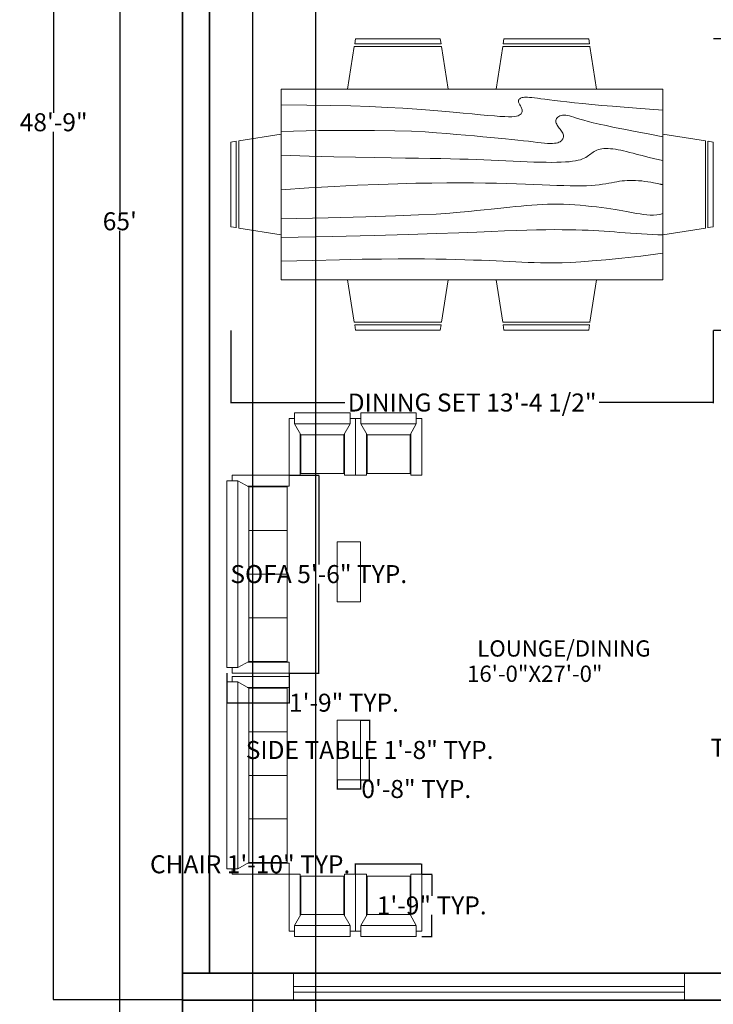
# Model space of a CAD drawing. Units: inches. Extents: x 79 to 8696167, y -3690578 to 147.
# Tile 2 of 10: x 79 to 310, y -551 to -223. Entities that reach past the tile are written whole.
import ezdxf

# ---------------------------------------------------------------- set-up
doc = ezdxf.new("R2010")
doc.units = ezdxf.units.IN
doc.header["$MEASUREMENT"] = 0
doc.layers.get('0').update_dxf_attribs({"color": 253})
for name, color, linetype, lineweight in [('A-ANNO-DIMS', 2, 'Continuous', 18), ('A-AREA-IDEN', 7, 'Continuous', 18), ('C-PROP', 7, 'Continuous', 35), ('furniture', 30, 'Continuous', 18), ('walls', 8, 'Continuous', 35), ('windows', 171, 'Continuous', 18)]:
    doc.layers.add(name, color=color, linetype=linetype, lineweight=lineweight)
doc.styles.get("Standard").update_dxf_attribs({"font": 'arial.ttf'})
doc.dimstyles.get("Standard").update_dxf_attribs({"dimtxt": 6, "dimasz": 0.18, "dimexe": 0.18, "dimexo": 0.0625, "dimgap": 0.09, "dimtad": 0, "dimtih": 1, "dimtoh": 1, "dimzin": 0, "dimdsep": 46, "dimlunit": 3, "dimtxsty": 'Standard', "dimcen": 0.09, "dimadec": 0, "dimazin": 0, "dimtfac": 1, "dimtofl": 0, "dimtmove": 0, "dimatfit": 3, "dimfxl": 1, "dimtolj": 1, "dimtzin": 0, "dimarcsym": 0})

# ---------------------------------------------------------------- blocks, each defined once
blk = doc.blocks.new('Dining Set - 36 x 72 in.')
for p, q in [((-22, 27.5), (-22.1562, 26.50042)), ((-5.8416, 26.5), (-22.1534, 26.5)), ((-22, 27.5), (-6, 27.5)), ((-5.8437, 26.49966), (-6, 27.5)), ((6, 27.5), (5.8438, 26.50042)), ((22.1584, 26.5), (5.8466, 26.5)), ((6, 27.5), (22, 27.5)), ((22.1563, 26.49966), (22, 27.5)), ((-22.2343, 26.00059), (-23.4847, 17.99762)), ((-22.2304, 26), (-5.7608, 26)), ((-4.5152, 17.99762), (-5.7655, 25.99926)), ((5.7657, 26.00059), (4.5153, 17.99762)), ((5.7696, 26), (22.2392, 26)), ((23.4848, 17.99762), (22.2345, 25.99926)), ((36, 18), (-36, 18)), ((-36, 18), (-36, -18)), ((36, -18), (36, 18)), ((-44.0006, 8.23428), (-35.9976, 9.48474)), ((44.0006, 8.23428), (35.9976, 9.48474)), ((-45.5, 8), (-44.5004, 8.15617)), ((-45.5, 8), (-45.5, -8)), ((-44.5, -8.15843), (-44.5, 8.15338)), ((-44, 8.23041), (-44, -8.23915)), ((44, 8.23041), (44, -8.23915)), ((44.5, -8.15843), (44.5, 8.15338)), ((45.5, 8), (44.5005, 8.15617)), ((45.5, 8), (45.5, -8)), ((-44.4997, -8.15631), (-45.5, -8)), ((-35.9976, -9.48476), (-43.9993, -8.2345)), ((35.9976, -9.48476), (43.9993, -8.2345)), ((44.4997, -8.15631), (45.5, -8)), ((-36, -18), (36, -18)), ((-22.2343, -26.0006), (-23.4847, -17.99762)), ((-4.5152, -17.99762), (-5.7655, -25.99928)), ((5.7657, -26.0006), (4.5153, -17.99762)), ((23.4848, -17.99762), (22.2345, -25.99928)), ((-22.2304, -26), (-5.7608, -26)), ((5.7696, -26), (22.2392, -26)), ((-22, -27.5), (-22.1562, -26.50044)), ((-5.8416, -26.5), (-22.1534, -26.5)), ((-22, -27.5), (-6, -27.5)), ((-5.8437, -26.49967), (-6, -27.5)), ((6, -27.5), (5.8438, -26.50044)), ((22.1584, -26.5), (5.8466, -26.5)), ((6, -27.5), (22, -27.5)), ((22.1563, -26.49967), (22, -27.5))]:
    blk.add_line(p, q)
for points in [[(-36, 15), (-31.1772, 14.97754), (-26.8079, 14.91406), (-22.8538, 14.81543), (-19.276, 14.6875), (-16.0362, 14.53613), (-13.0957, 14.36718), (-10.4159, 14.18652), (-7.9583, 14), (-5.6904, 13.81315), (-3.6035, 13.63021), (-1.6954, 13.45508), (0.0365, 13.29166), (1.5945, 13.14388), (2.9811, 13.01562), (4.1988, 12.9108), (5.25, 12.83333), (6.1393, 12.78613), (6.8802, 12.76823), (7.4883, 12.77767), (7.9792, 12.8125), (8.3685, 12.87077), (8.6719, 12.95052), (8.9049, 13.0498), (9.0833, 13.16666), (9.2205, 13.29899), (9.3216, 13.44401), (9.3895, 13.59879), (9.4271, 13.76041), (9.4373, 13.92594), (9.4232, 14.09245), (9.3875, 14.257), (9.3333, 14.41666), (9.2638, 14.56917), (9.1836, 14.71484), (9.0975, 14.85465), (9.0104, 14.98958), (8.9272, 15.1206), (8.8529, 15.2487), (8.7922, 15.37483), (8.75, 15.5), (8.7305, 15.62467), (8.7344, 15.74739), (8.7617, 15.86621), (8.8125, 15.97916), (8.8867, 16.08431), (8.9844, 16.17968), (9.1055, 16.26334), (9.25, 16.33333), (9.4189, 16.38802), (9.6172, 16.42708), (9.8506, 16.45052), (10.125, 16.45833), (10.4463, 16.45052), (10.8203, 16.42708), (11.2529, 16.38802), (11.75, 16.33333), (12.3184, 16.26318), (12.9694, 16.17838), (13.7151, 16.07991), (14.5677, 15.96875), (15.5395, 15.84586), (16.6426, 15.71224), (17.8893, 15.56884), (19.2917, 15.41666), (20.859, 15.25667), (22.5879, 15.08984), (24.4721, 14.91715), (26.5052, 14.73958), (28.6809, 14.5581), (30.9929, 14.3737), (33.4347, 14.18733), (36, 14)], [(-36, 10), (-28.9766, 10.14274), (-23.1725, 10.20442), (-18.4241, 10.19775), (-14.5677, 10.13541), (-11.4399, 10.03011), (-8.877, 9.89453), (-6.7154, 9.74137), (-4.7917, 9.58333), (-2.9698, 9.43082), (-1.2246, 9.28515), (0.4415, 9.14534), (2.026, 9.01041), (3.5266, 8.87939), (4.9408, 8.7513), (6.266, 8.62516), (7.5, 8.5), (8.6411, 8.37549), (9.6914, 8.2539), (10.6538, 8.13818), (11.5312, 8.03125), (12.3267, 7.93603), (13.043, 7.85547), (13.6831, 7.79248), (14.25, 7.75), (14.7471, 7.7303), (15.1797, 7.73307), (15.5537, 7.75732), (15.875, 7.80208), (16.1494, 7.86637), (16.3828, 7.94922), (16.5811, 8.04964), (16.75, 8.16666), (16.8944, 8.29915), (17.0143, 8.44531), (17.1089, 8.60319), (17.1771, 8.77083), (17.218, 8.94629), (17.2305, 9.1276), (17.2137, 9.31282), (17.1667, 9.5), (17.0895, 9.6875), (16.987, 9.875), (16.8649, 10.0625), (16.7292, 10.25), (16.5856, 10.4375), (16.4401, 10.625), (16.2985, 10.8125), (16.1667, 11), (16.05, 11.18733), (15.9518, 11.3737), (15.8752, 11.5581), (15.8229, 11.73958), (15.798, 11.91715), (15.8034, 12.08984), (15.842, 12.25667), (15.9167, 12.41666), (16.0295, 12.56836), (16.1784, 12.70833), (16.3605, 12.83268), (16.5729, 12.9375), (16.8127, 13.01888), (17.0768, 13.07291), (17.3625, 13.0957), (17.6667, 13.08333), (17.9894, 13.03312), (18.3418, 12.94726), (18.7382, 12.82918), (19.1927, 12.68229), (19.7195, 12.51001), (20.3327, 12.31575), (21.0465, 12.10294), (21.875, 11.875), (22.8357, 11.63354), (23.959, 11.37304), (25.2786, 11.08618), (26.8282, 10.76562), (28.6414, 10.40405), (30.752, 9.99414), (33.1936, 9.52856), (36, 9)], [(-36, 5.5), (-30.7157, 5.3348), (-26.069, 5.20963), (-21.9946, 5.11767), (-18.4271, 5.05208), (-15.3009, 5.00602), (-12.5508, 4.97265), (-10.1112, 4.94515), (-7.9167, 4.91666), (-5.909, 4.88167), (-4.0586, 4.83984), (-2.3429, 4.79215), (-0.7396, 4.73958), (0.7739, 4.6831), (2.22, 4.6237), (3.6213, 4.56233), (5, 4.5), (6.373, 4.43782), (7.7344, 4.3776), (9.0723, 4.32129), (10.375, 4.27083), (11.6309, 4.22819), (12.8281, 4.19531), (13.9551, 4.17415), (15, 4.16666), (15.954, 4.17448), (16.819, 4.19791), (17.6001, 4.23698), (18.3021, 4.29166), (18.9299, 4.36198), (19.4883, 4.44791), (19.9823, 4.54948), (20.4167, 4.66666), (20.7969, 4.79899), (21.1302, 4.94401), (21.4245, 5.09879), (21.6875, 5.26041), (21.9271, 5.42594), (22.1511, 5.59245), (22.3672, 5.757), (22.5834, 5.91666), (22.8065, 6.06868), (23.0404, 6.21093), (23.2879, 6.34147), (23.5521, 6.45833), (23.8358, 6.55957), (24.142, 6.64323), (24.4735, 6.70735), (24.8334, 6.75), (25.2235, 6.76969), (25.642, 6.76692), (26.0858, 6.74267), (26.5521, 6.69791), (27.0379, 6.63362), (27.5404, 6.55078), (28.0565, 6.45036), (28.5834, 6.33333), (29.1242, 6.19987), (29.7071, 6.04687), (30.3661, 5.87044), (31.1354, 5.66666), (32.0493, 5.43164), (33.142, 5.16146), (34.4475, 4.85221), (36, 4.5)], [(-36, -1), (-30.7915, -0.6591), (-26.0195, -0.38216), (-21.6519, -0.16284), (-17.6563, 0.00521), (-14.0005, 0.12833), (-10.6523, 0.21289), (-7.5796, 0.26522), (-4.75, 0.29166), (-2.134, 0.29793), (0.2878, 0.28711), (2.5317, 0.26163), (4.6146, 0.22396), (6.5529, 0.17651), (8.3633, 0.12174), (10.0623, 0.06209), (11.6667, 0), (13.1899, -0.06201), (14.6341, -0.1211), (15.9982, -0.17432), (17.2813, -0.21875), (18.4823, -0.25147), (19.6003, -0.26953), (20.6343, -0.27002), (21.5834, -0.25), (22.4481, -0.20768), (23.2357, -0.14584), (23.9549, -0.06836), (24.6146, 0.02083), (25.2235, 0.11784), (25.7904, 0.21875), (26.3241, 0.31966), (26.8334, 0.41666), (27.3265, 0.50618), (27.8099, 0.58593), (28.2894, 0.65397), (28.7709, 0.70833), (29.2601, 0.74707), (29.763, 0.76823), (30.2855, 0.76985), (30.8334, 0.75), (31.4088, 0.70784), (31.9994, 0.64713), (32.589, 0.57275), (33.1615, 0.48958), (33.7008, 0.4025), (34.1908, 0.3164), (34.6153, 0.23616), (34.9584, 0.16666), (35.2099, 0.11165), (35.3848, 0.07031), (35.504, 0.04069), (35.5886, 0.02083), (35.6594, 0.00879), (35.7377, 0.0026), (35.8442, 0.00032), (36, 0)], [(-36, -6.5), (-27.1843, -6.31267), (-20.084, -6.1263), (-14.469, -5.9419), (-10.1094, -5.76042), (-6.7752, -5.58285), (-4.2363, -5.41016), (-2.2629, -5.24333), (-0.625, -5.08334), (0.8708, -4.93099), (2.2715, -4.78646), (3.5872, -4.64974), (4.8281, -4.52084), (6.0046, -4.39974), (7.127, -4.28646), (8.2053, -4.18099), (9.25, -4.08334), (10.2705, -3.99382), (11.2734, -3.91407), (12.2647, -3.84603), (13.25, -3.79167), (14.2354, -3.75293), (15.2266, -3.73177), (16.2295, -3.73015), (17.25, -3.75), (18.2912, -3.79248), (19.3451, -3.85547), (20.4009, -3.93604), (21.4479, -4.03125), (22.4754, -4.13819), (23.4727, -4.25391), (24.4289, -4.37549), (25.3334, -4.5), (26.1785, -4.62492), (26.9694, -4.74935), (27.7145, -4.87281), (28.4219, -4.99479), (29.1, -5.11483), (29.7572, -5.23242), (30.4016, -5.34709), (31.0417, -5.45834), (31.6837, -5.56437), (32.3262, -5.65821), (32.9658, -5.73153), (33.599, -5.77604), (34.2224, -5.78345), (34.8327, -5.74545), (35.4264, -5.65373), (36, -5.5)], [(-36, -10), (-26.4022, -9.81299), (-18.4675, -9.62891), (-11.9839, -9.45069), (-6.7396, -9.28125), (-2.5226, -9.12354), (0.8789, -8.98047), (3.6769, -8.85498), (6.0833, -8.75), (8.2767, -8.66765), (10.3021, -8.60677), (12.1712, -8.56543), (13.8958, -8.54167), (15.4876, -8.53353), (16.9583, -8.53907), (18.3197, -8.55632), (19.5834, -8.58334), (20.7616, -8.61841), (21.8685, -8.66081), (22.9188, -8.71004), (23.9271, -8.76563), (24.9081, -8.82707), (25.8763, -8.89388), (26.8465, -8.96558), (27.8334, -9.04167), (28.8474, -9.12118), (29.8828, -9.20117), (30.93, -9.27824), (31.9792, -9.34896), (33.0205, -9.40991), (34.0443, -9.45768), (35.0407, -9.48885), (36, -9.5)], [(-36, -14.5), (-30.0881, -14.33513), (-25.0332, -14.21224), (-20.7312, -14.12647), (-17.0781, -14.07292), (-13.97, -14.04671), (-11.3027, -14.04297), (-8.9724, -14.05681), (-6.875, -14.08334), (-4.9224, -14.11833), (-3.0905, -14.16016), (-1.3709, -14.20785), (0.2448, -14.26042), (1.7647, -14.3169), (3.1973, -14.3763), (4.5507, -14.43767), (5.8333, -14.5), (7.0554, -14.5621), (8.235, -14.62175), (9.3922, -14.67652), (10.5469, -14.72396), (11.7192, -14.76164), (12.929, -14.78711), (14.1965, -14.79794), (15.5417, -14.79167), (16.9933, -14.76424), (18.6152, -14.70508), (20.4804, -14.60197), (22.6615, -14.44271), (25.2312, -14.21509), (28.2624, -13.9069), (31.8277, -13.50594), (36, -13)]]:
    blk.add_lwpolyline(points)
blk = doc.blocks.new('FABRIC SOFA 4S')
at = {"layer": 'furniture'}
for p, q in [((3, 54), (34, 54)), ((3, 51), (3, 54)), ((34, 48), (34, 54)), ((0, -51), (0, 51)), ((6, 51), (0, 51)), ((6, -51), (6, 51)), ((12, 47.63), (6, 51)), ((11.14, 48), (34, 48)), ((33, 23.81), (12, 23.81)), ((33, 0), (12, 0)), ((33, -23.81), (12, -23.81)), ((6, -51), (12, -47.63)), ((11.54, -48), (34, -48)), ((34, -48), (34, -54)), ((6, -51), (0, -51)), ((3, -54), (3, -51)), ((3, -54), (34, -54))]:
    blk.add_line(p, q, dxfattribs=at)
blk.add_lwpolyline([(12, -47.63), (12, 47.63), (33, 47.63), (33, -47.63)], close=True, dxfattribs=at)
blk = doc.blocks.new('FABRIC SOFA 1S')
at = {"layer": 'furniture'}
for p, q in [((3, 18.12), (34, 18.12)), ((3, 15.12), (3, 18.12)), ((34, 12.12), (34, 18.12)), ((0, -15.12), (0, 15.12)), ((6, 15.12), (0, 15.12)), ((6, -15.12), (6, 15.12)), ((12, 11.75), (6, 15.12)), ((11.33, 12.12), (34, 12.12)), ((6, -15.12), (0, -15.12)), ((3, -18.12), (3, -15.12)), ((6, -15.12), (12, -11.75)), ((11.33, -12.12), (34, -12.12)), ((34, -12.12), (34, -18.12)), ((3, -18.12), (34, -18.12))]:
    blk.add_line(p, q, dxfattribs=at)
blk.add_lwpolyline([(12, -11.75), (12, 11.75), (33, 11.75), (33, -11.75)], close=True, dxfattribs=at)
blk = doc.blocks.new('*D23')
at = {"layer": 'A-ANNO-DIMS', "color": 0, "lineweight": -2, "transparency": 16777216}
for p, q in [((133.38, 99.88), (112.4, 99.88)), ((112.58, 99.7), (112.58, -286.97)), ((112.58, -679.94), (112.58, -293.28)), ((133.38, -680.12), (112.4, -680.12))]:
    blk.add_line(p, q, dxfattribs=at)
at = {"layer": 'A-ANNO-DIMS', "color": 0, "lineweight": 100, "transparency": 16777216}
for points in [[(112.55, 99.7), (112.61, 99.7), (112.58, 99.88)], [(112.55, -679.94), (112.61, -679.94), (112.58, -680.12)]]:
    blk.add_solid(points, dxfattribs=at)
at = {"layer": 'Defpoints', "color": 0, "lineweight": 100, "transparency": 16777216}
for p in [(112.58, 99.88), (133.44, 99.88), (133.44, -680.12)]:
    blk.add_point(p, dxfattribs=at)
at = {"layer": 'A-ANNO-DIMS', "color": 0, "transparency": 16777216, "insert": (112.58, -290.12), "char_height": 6, "attachment_point": 5}
blk.add_mtext("\\A1;65'", dxfattribs=at)
blk = doc.blocks.new('TABLE-LOUNGE-NARROW')
for p, q in [((0, 19.98), (7.85, 19.98)), ((0, 0), (0, 19.98)), ((7.85, 19.98), (7.85, 0)), ((7.85, 0), (0, 0))]:
    blk.add_line(p, q)
blk = doc.blocks.new('*D33')
at = {"layer": 'A-ANNO-DIMS', "color": 0, "lineweight": -2, "transparency": 16777216}
for p, q in [((191.08, -504.4), (190.9, -504.4)), ((191.08, -507.66), (191.08, -504.22)), ((213.03, -504.4), (191.26, -504.4)), ((213.21, -507.66), (213.21, -504.22))]:
    blk.add_line(p, q, dxfattribs=at)
at = {"layer": 'A-ANNO-DIMS', "color": 0, "lineweight": 100, "transparency": 16777216}
for points in [[(191.26, -504.37), (191.26, -504.43), (191.08, -504.4)], [(213.03, -504.37), (213.03, -504.43), (213.21, -504.4)]]:
    blk.add_solid(points, dxfattribs=at)
at = {"layer": 'Defpoints', "color": 0, "lineweight": 100, "transparency": 16777216}
for p in [(191.08, -504.4), (191.08, -507.72), (213.21, -507.72)]:
    blk.add_point(p, dxfattribs=at)
at = {"layer": 'A-ANNO-DIMS', "color": 0, "transparency": 16777216, "insert": (156.02, -504.4), "char_height": 6, "attachment_point": 5}
blk.add_mtext('\\A1;CHAIR 1\'-10" TYP.', dxfattribs=at)
blk = doc.blocks.new('*D34')
at = {"layer": 'A-ANNO-DIMS', "color": 0, "lineweight": -2, "transparency": 16777216}
for p, q in [((213.27, -507.72), (216.71, -507.72)), ((216.53, -507.9), (216.53, -514.95)), ((216.53, -528.3), (216.53, -521.25)), ((213.27, -528.48), (216.71, -528.48))]:
    blk.add_line(p, q, dxfattribs=at)
at = {"layer": 'A-ANNO-DIMS', "color": 0, "lineweight": 100, "transparency": 16777216}
for points in [[(216.5, -507.9), (216.56, -507.9), (216.53, -507.72)], [(216.5, -528.3), (216.56, -528.3), (216.53, -528.48)]]:
    blk.add_solid(points, dxfattribs=at)
at = {"layer": 'Defpoints', "color": 0, "lineweight": 100, "transparency": 16777216}
for p in [(213.21, -507.72), (216.53, -507.72), (213.21, -528.48)]:
    blk.add_point(p, dxfattribs=at)
at = {"layer": 'A-ANNO-DIMS', "color": 0, "transparency": 16777216, "insert": (216.53, -518.1), "char_height": 6, "attachment_point": 5}
blk.add_mtext('\\A1;1\'-9" TYP.', dxfattribs=at)
blk = doc.blocks.new('*D35')
at = {"layer": 'A-ANNO-DIMS', "color": 0, "lineweight": -2, "transparency": 16777216}
for p, q in [((169.07, -374.73), (179.07, -374.73)), ((178.89, -374.91), (178.89, -404.5)), ((178.89, -440.48), (178.89, -410.89)), ((169.07, -440.66), (179.07, -440.66))]:
    blk.add_line(p, q, dxfattribs=at)
at = {"layer": 'A-ANNO-DIMS', "color": 0, "lineweight": 100, "transparency": 16777216}
for points in [[(178.86, -374.91), (178.92, -374.91), (178.89, -374.73)], [(178.86, -440.48), (178.92, -440.48), (178.89, -440.66)]]:
    blk.add_solid(points, dxfattribs=at)
at = {"layer": 'Defpoints', "color": 0, "lineweight": 100, "transparency": 16777216}
for p in [(169, -374.73), (178.89, -374.73), (169, -440.66)]:
    blk.add_point(p, dxfattribs=at)
at = {"layer": 'A-ANNO-DIMS', "color": 0, "transparency": 16777216, "insert": (178.89, -407.69), "char_height": 6, "attachment_point": 5}
blk.add_mtext('\\A1;SOFA 5\'-6" TYP.', dxfattribs=at)
blk = doc.blocks.new('*D36')
at = {"layer": 'A-ANNO-DIMS', "color": 0, "lineweight": -2, "transparency": 16777216}
for p, q in [((148.25, -440.72), (148.25, -450.73)), ((169, -440.72), (169, -450.73)), ((148.43, -450.55), (168.82, -450.55)), ((169, -450.55), (169.18, -450.55))]:
    blk.add_line(p, q, dxfattribs=at)
at = {"layer": 'A-ANNO-DIMS', "color": 0, "lineweight": 100, "transparency": 16777216}
for points in [[(148.43, -450.52), (148.43, -450.58), (148.25, -450.55)], [(168.82, -450.52), (168.82, -450.58), (169, -450.55)]]:
    blk.add_solid(points, dxfattribs=at)
at = {"layer": 'Defpoints', "color": 0, "lineweight": 100, "transparency": 16777216}
for p in [(148.25, -440.66), (169, -440.66), (169, -450.55)]:
    blk.add_point(p, dxfattribs=at)
at = {"layer": 'A-ANNO-DIMS', "color": 0, "transparency": 16777216, "insert": (187.28, -450.55), "char_height": 6, "attachment_point": 5}
blk.add_mtext('\\A1;1\'-9" TYP.', dxfattribs=at)
blk = doc.blocks.new('*D37')
at = {"layer": 'A-ANNO-DIMS', "color": 0, "lineweight": -2, "transparency": 16777216}
for p, q in [((192.89, -456.32), (196.01, -456.32)), ((195.83, -456.5), (195.83, -463.12)), ((195.83, -476.12), (195.83, -469.5)), ((192.89, -476.3), (196.01, -476.3))]:
    blk.add_line(p, q, dxfattribs=at)
at = {"layer": 'A-ANNO-DIMS', "color": 0, "lineweight": 100, "transparency": 16777216}
for points in [[(195.8, -456.5), (195.86, -456.5), (195.83, -456.32)], [(195.8, -476.12), (195.86, -476.12), (195.83, -476.3)]]:
    blk.add_solid(points, dxfattribs=at)
at = {"layer": 'Defpoints', "color": 0, "lineweight": 100, "transparency": 16777216}
for p in [(192.83, -456.32), (195.83, -456.32), (192.83, -476.3)]:
    blk.add_point(p, dxfattribs=at)
at = {"layer": 'A-ANNO-DIMS', "color": 0, "transparency": 16777216, "insert": (195.83, -466.31), "char_height": 6, "attachment_point": 5}
blk.add_mtext('\\A1;SIDE TABLE 1\'-8" TYP.', dxfattribs=at)
blk = doc.blocks.new('*D38')
at = {"layer": 'A-ANNO-DIMS', "color": 0, "lineweight": -2, "transparency": 16777216}
for p, q in [((184.98, -476.36), (184.98, -479.48)), ((192.83, -476.36), (192.83, -479.48)), ((185.16, -479.3), (192.65, -479.3)), ((192.83, -479.3), (193.01, -479.3))]:
    blk.add_line(p, q, dxfattribs=at)
at = {"layer": 'A-ANNO-DIMS', "color": 0, "lineweight": 100, "transparency": 16777216}
for points in [[(185.16, -479.27), (185.16, -479.33), (184.98, -479.3)], [(192.65, -479.27), (192.65, -479.33), (192.83, -479.3)]]:
    blk.add_solid(points, dxfattribs=at)
at = {"layer": 'Defpoints', "color": 0, "lineweight": 100, "transparency": 16777216}
for p in [(184.98, -476.3), (192.83, -476.3), (192.83, -479.3)]:
    blk.add_point(p, dxfattribs=at)
at = {"layer": 'A-ANNO-DIMS', "color": 0, "transparency": 16777216, "insert": (211.38, -479.3), "char_height": 6, "attachment_point": 5}
blk.add_mtext('\\A1;0\'-8" TYP.', dxfattribs=at)
blk = doc.blocks.new('*D39')
at = {"layer": 'A-ANNO-DIMS', "color": 0, "lineweight": -2, "transparency": 16777216}
for p, q in [((334.5, -445.33), (340.68, -445.33)), ((340.5, -445.51), (340.51, -462.36)), ((340.51, -485.59), (340.51, -468.75)), ((334.51, -485.77), (340.69, -485.77))]:
    blk.add_line(p, q, dxfattribs=at)
at = {"layer": 'A-ANNO-DIMS', "color": 0, "lineweight": 100, "transparency": 16777216}
for points in [[(340.53, -445.51), (340.47, -445.51), (340.5, -445.33)], [(340.54, -485.59), (340.48, -485.59), (340.51, -485.77)]]:
    blk.add_solid(points, dxfattribs=at)
at = {"layer": 'Defpoints', "color": 0, "lineweight": 100, "transparency": 16777216}
for p in [(334.44, -445.33), (340.5, -445.33), (334.44, -485.77)]:
    blk.add_point(p, dxfattribs=at)
at = {"layer": 'A-ANNO-DIMS', "color": 0, "transparency": 16777216, "insert": (340.51, -465.55), "char_height": 6, "attachment_point": 5}
blk.add_mtext('\\A1;TV 3\'-4 1/2" TYP.', dxfattribs=at)
blk = doc.blocks.new('*D51')
at = {"layer": 'A-ANNO-DIMS', "color": 0, "lineweight": -2, "transparency": 16777216}
for p, q in [((149.63, -326.48), (149.63, -350.7)), ((310.36, -326.48), (310.36, -350.7)), ((149.81, -350.52), (187.61, -350.52)), ((310.18, -350.52), (272.38, -350.52))]:
    blk.add_line(p, q, dxfattribs=at)
at = {"layer": 'A-ANNO-DIMS', "color": 0, "lineweight": 100, "transparency": 16777216}
for points in [[(149.81, -350.49), (149.81, -350.55), (149.63, -350.52)], [(310.18, -350.49), (310.18, -350.55), (310.36, -350.52)]]:
    blk.add_solid(points, dxfattribs=at)
at = {"layer": 'Defpoints', "color": 0, "lineweight": 100, "transparency": 16777216}
for p in [(149.63, -326.42), (310.36, -326.42), (310.36, -350.52)]:
    blk.add_point(p, dxfattribs=at)
at = {"layer": 'A-ANNO-DIMS', "color": 0, "transparency": 16777216, "insert": (229.99, -350.52), "char_height": 6, "attachment_point": 5}
blk.add_mtext('\\A1;DINING SET 13\'-4 1/2"', dxfattribs=at)
blk = doc.blocks.new('*D52')
at = {"layer": 'A-ANNO-DIMS', "color": 0, "lineweight": -2, "transparency": 16777216}
for p, q in [((310.42, -229.27), (334.65, -229.27)), ((334.47, -229.45), (334.47, -274.69)), ((334.47, -326.24), (334.47, -281)), ((310.42, -326.42), (334.65, -326.42))]:
    blk.add_line(p, q, dxfattribs=at)
at = {"layer": 'A-ANNO-DIMS', "color": 0, "lineweight": 100, "transparency": 16777216}
for points in [[(334.44, -229.45), (334.5, -229.45), (334.47, -229.27)], [(334.44, -326.24), (334.5, -326.24), (334.47, -326.42)]]:
    blk.add_solid(points, dxfattribs=at)
at = {"layer": 'Defpoints', "color": 0, "lineweight": 100, "transparency": 16777216}
for p in [(310.36, -229.27), (334.47, -229.27), (310.36, -326.42)]:
    blk.add_point(p, dxfattribs=at)
at = {"layer": 'A-ANNO-DIMS', "color": 0, "transparency": 16777216, "insert": (334.47, -277.84), "char_height": 6, "attachment_point": 5}
blk.add_mtext('\\A1;8\'-1"', dxfattribs=at)
blk = doc.blocks.new('*D56')
at = {"layer": 'A-ANNO-DIMS', "color": 0, "lineweight": -2, "transparency": 16777216}
for p, q in [((133.38, 35.38), (90.36, 35.38)), ((90.54, 35.2), (90.54, -253.97)), ((90.54, -549.44), (90.54, -260.28)), ((133.38, -549.62), (90.36, -549.62))]:
    blk.add_line(p, q, dxfattribs=at)
at = {"layer": 'A-ANNO-DIMS', "color": 0, "lineweight": 100, "transparency": 16777216}
for points in [[(90.51, 35.2), (90.57, 35.2), (90.54, 35.38)], [(90.51, -549.44), (90.57, -549.44), (90.54, -549.62)]]:
    blk.add_solid(points, dxfattribs=at)
at = {"layer": 'Defpoints', "color": 0, "lineweight": 100, "transparency": 16777216}
for p in [(90.54, 35.38), (133.44, 35.38), (133.44, -549.62)]:
    blk.add_point(p, dxfattribs=at)
at = {"layer": 'A-ANNO-DIMS', "color": 0, "transparency": 16777216, "insert": (90.54, -257.12), "char_height": 6, "attachment_point": 5}
blk.add_mtext('\\A1;48\'-9"', dxfattribs=at)
blk = doc.blocks.new('*D59')
at = {"layer": 'A-ANNO-DIMS', "color": 0, "lineweight": -2, "transparency": 16777216}
for p, q in [((156.82, 2.31), (156.82, -723.2)), ((177.82, 2.31), (177.82, -723.2)), ((157, -723.02), (159.53, -723.02)), ((177.64, -723.02), (175.1, -723.02))]:
    blk.add_line(p, q, dxfattribs=at)
at = {"layer": 'A-ANNO-DIMS', "color": 0, "lineweight": 100, "transparency": 16777216}
for points in [[(157, -722.99), (157, -723.05), (156.82, -723.02)], [(177.64, -722.99), (177.64, -723.05), (177.82, -723.02)]]:
    blk.add_solid(points, dxfattribs=at)
at = {"layer": 'Defpoints', "color": 0, "lineweight": 100, "transparency": 16777216}
for p in [(156.82, 2.38), (177.82, 2.38), (177.82, -723.02)]:
    blk.add_point(p, dxfattribs=at)
at = {"layer": 'A-ANNO-DIMS', "color": 0, "transparency": 16777216, "insert": (167.32, -723.02), "char_height": 6, "attachment_point": 5}
blk.add_mtext('\\A1;1\'-9"', dxfattribs=at)

msp = doc.modelspace()

# ---------------------------------------------------------------- linework, layer by layer
at = {"layer": 'C-PROP'}
msp.add_line((133.441, -680.125), (133.441, 99.875), dxfattribs=at)
at = {"layer": 'walls'}
for p, q in [((142.441, -540.625), (142.441, -216.625)), ((133.441, -540.625), (334.441, -540.625)), ((133.441, -549.625), (343.441, -549.625))]:
    msp.add_line(p, q, dxfattribs=at)
at = {"layer": 'windows'}
for p, q in [((170.416, -540.625), (170.416, -549.625)), ((300.715, -540.625), (170.416, -540.625)), ((170.416, -540.625), (170.416, -545.125)), ((300.715, -549.625), (300.715, -540.625)), ((170.416, -545.125), (300.715, -545.125)), ((300.715, -547.026), (170.416, -547.026)), ((300.715, -545.125), (300.715, -547.026)), ((170.416, -549.625), (300.715, -549.625))]:
    msp.add_line(p, q, dxfattribs=at)

# ---------------------------------------------------------------- block references
at = {"layer": 'furniture'}
for name, p, xscale, yscale, zscale in [('Dining Set - 36 x 72 in.', (229.994, -277.843), 1.766251471403308, 1.766251471403308, 1.766251471403308), ('FABRIC SOFA 4S', (148.249, -407.694), 0.6104321447770836, 0.6104321447770836, 0.6104321447770836), ('FABRIC SOFA 4S', (148.249, -474.758), 0.6104321447770836, 0.6104321447770836, 0.6104321447770836)]:
    msp.add_blockref(name, p, dxfattribs=dict(at, xscale=xscale, yscale=yscale, zscale=zscale))
at = {"layer": 'furniture', "yscale": 0.6104321447770836, "zscale": 0.6104321447770836, "rotation": 90}
for p, xscale in [((180.067, -353.976), -0.6104321447770836), ((202.144, -353.976), -0.6104321447770836), ((180.067, -528.476), 0.6104321447770836), ((202.144, -528.476), 0.6104321447770836)]:
    msp.add_blockref('FABRIC SOFA 1S', p, dxfattribs=dict(at, xscale=xscale))
at = {"layer": 'furniture'}
for p in [(184.978, -416.898), (184.978, -476.301)]:
    msp.add_blockref('TABLE-LOUNGE-NARROW', p, dxfattribs=at)

# ---------------------------------------------------------------- texts
at = {"layer": 'A-AREA-IDEN'}
for s, p in [('LOUNGE/DINING', (231.691, -435.19)), ('16\'-0"X27\'-0"', (228.299, -443.616))]:
    msp.add_text(s, height=5.42229, dxfattribs=at).set_placement(p)

# ---------------------------------------------------------------- dimensions: what is measured, and where the dimension line sits
at = {"layer": 'A-ANNO-DIMS'}
for base, p1, p2, override, picture, middle in [((112.58, 99.875), (133.441, -680.125), (133.441, 99.875), {"dimclrd": 0, "dimclre": 0, "dimclrt": 0}, '*D23', (112.58, -290.125)), ((90.541, 35.375), (133.441, -549.625), (133.441, 35.375), {"dimdec": 1, "dimlfac": 1, "dimrnd": 0, "dimzin": 1, "dimdsep": 46, "dimlunit": 4, "dimfrac": 2}, '*D56', (90.541, -257.125)), ((334.468, -229.271), (310.359, -326.415), (310.359, -229.271), {"dimdec": 1, "dimlfac": 1, "dimrnd": 0, "dimzin": 1, "dimdsep": 46, "dimlunit": 4, "dimfrac": 2}, '*D52', (334.468, -277.843))]:
    dim = msp.add_linear_dim(base=base, p1=p1, p2=p2, angle=90, dimstyle='Standard', override=override, dxfattribs=at)
    dim.commit()
    dim.dimension.update_dxf_attribs({"geometry": picture, "text_midpoint": middle})
dim = msp.add_linear_dim(base=(177.817, -723.025), p1=(156.817, 2.375), p2=(177.817, 2.375), dimstyle='Standard', override={"dimdec": 1, "dimlfac": 1, "dimrnd": 0, "dimzin": 1, "dimdsep": 46, "dimlunit": 4, "dimfrac": 2}, dxfattribs=at)
dim.commit()
dim.dimension.update_dxf_attribs({"geometry": '*D59', "text_midpoint": (167.317, -723.025)})
for base, p1, p2, text, picture, middle in [((310.359, -350.524), (149.63, -326.415), (310.359, -326.415), 'DINING SET <>', '*D51', (229.994, -350.524)), ((169.003, -450.546), (148.249, -440.657), (169.003, -440.657), '<> TYP.', '*D36', (187.277, -450.546)), ((192.828, -479.2981), (184.9781, -476.3011), (192.828, -476.3011), '<> TYP.', '*D38', (211.3845, -479.2981))]:
    dim = msp.add_linear_dim(base=base, p1=p1, p2=p2, text=text, dimstyle='Standard', override={"dimdec": 1, "dimlfac": 1, "dimrnd": 0, "dimzin": 1, "dimdsep": 46, "dimlunit": 4, "dimfrac": 2}, dxfattribs=at)
    dim.commit()
    dim.dimension.update_dxf_attribs({"geometry": picture, "text_midpoint": middle})
for base, p1, p2, angle, text, picture, middle in [((178.892, -374.73), (169.003, -440.657), (169.003, -374.73), 90, 'SOFA <> TYP.', '*D35', (178.892, -407.694)), ((340.503, -445.331), (334.444, -485.772), (334.438, -445.332), 90.00902, 'TV <> TYP.', '*D39', (340.507, -465.551)), ((195.825, -456.321), (192.828, -476.301), (192.828, -456.321), 90, 'SIDE TABLE <> TYP.', '*D37', (195.825, -466.311)), ((191.08, -504.402), (213.208, -507.721), (191.08, -507.721), 180, 'CHAIR <> TYP.', '*D33', (156.023, -504.402)), ((216.527, -507.721), (213.208, -528.476), (213.208, -507.721), 90, '<> TYP.', '*D34', (216.527, -518.099))]:
    dim = msp.add_linear_dim(base=base, p1=p1, p2=p2, angle=angle, text=text, dimstyle='Standard', override={"dimdec": 1, "dimlfac": 1, "dimrnd": 0, "dimzin": 1, "dimdsep": 46, "dimlunit": 4, "dimfrac": 2}, dxfattribs=at)
    dim.commit()
    dim.dimension.update_dxf_attribs({"geometry": picture, "text_midpoint": middle})

doc.saveas('drawing.dxf')
